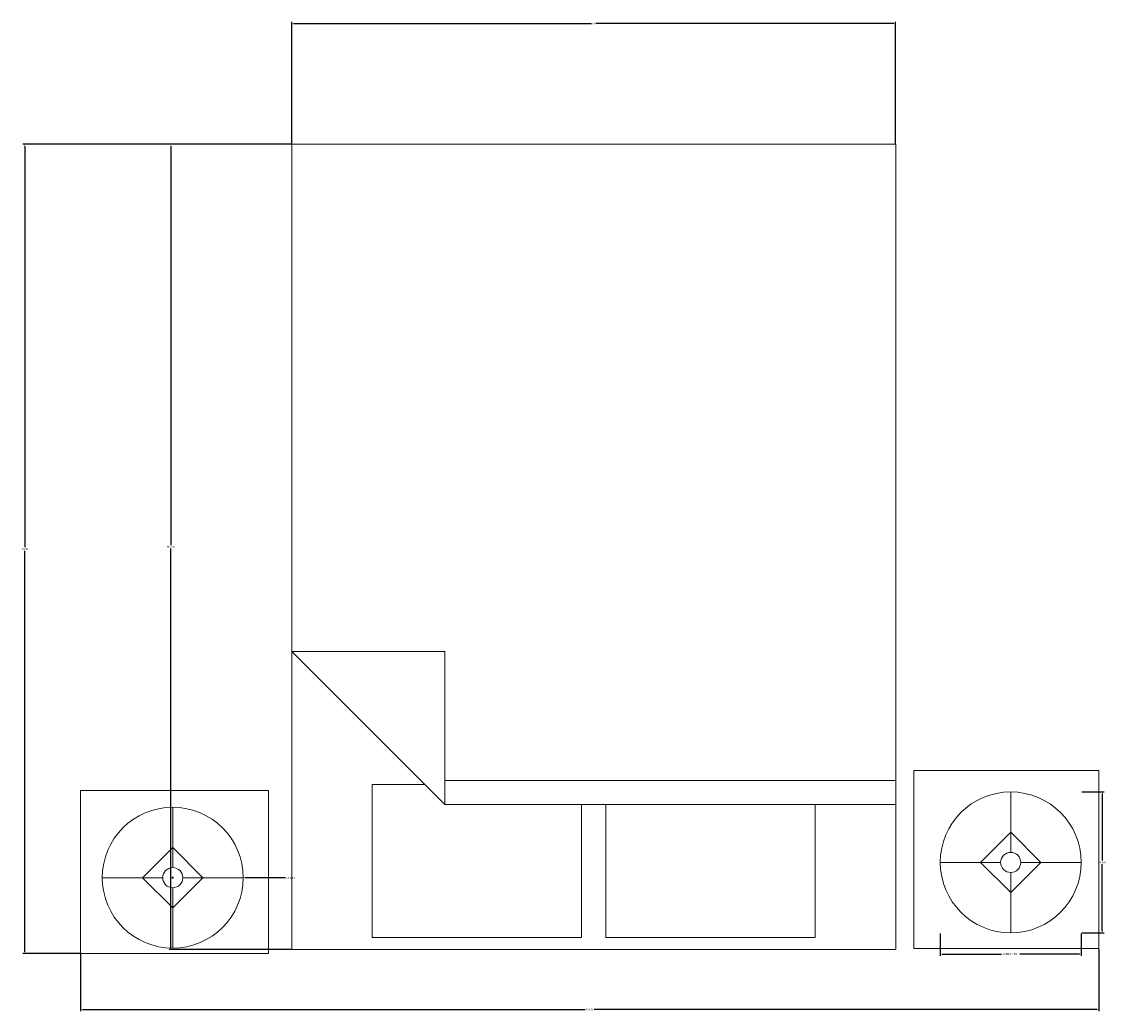
# Model space of a CAD drawing. Units: inches. Extents: x -52 to 1967, y 32 to 824.
# Tile 10 of 10: x 1859 to 1967, y 425 to 523. Entities that reach past the tile are written whole.
import ezdxf

# ---------------------------------------------------------------- set-up
doc = ezdxf.new("R2010")
doc.units = ezdxf.units.IN
doc.layers.add('A-ANNO-DIMS', color=2, linetype='Continuous', lineweight=18)
doc.layers.add('A-FURN', color=8, linetype='Continuous', lineweight=18)
doc.styles.get("Standard").update_dxf_attribs({"font": 'arial.ttf'})
doc.dimstyles.get("Standard").update_dxf_attribs({"dimtxt": 0.18, "dimasz": 0.18, "dimexe": 0.18, "dimexo": 0.0625, "dimgap": 0.09, "dimtad": 0, "dimtih": 1, "dimtoh": 1, "dimdec": 4, "dimzin": 0, "dimdsep": 46, "dimtxsty": 'Standard', "dimcen": 0.09, "dimadec": 0, "dimazin": 0, "dimtfac": 1, "dimtdec": 4, "dimtofl": 0, "dimtmove": 0, "dimatfit": 3, "dimfxl": 1, "dimtolj": 1, "dimtzin": 0, "dimarcsym": 0})

# ---------------------------------------------------------------- blocks, each defined once
blk = doc.blocks.new('Lamp - Table')
for p, q in [((0, 7), (0, 1)), ((0, 3), (-3, 0)), ((3, 0), (0, 3)), ((-1, 0), (-7, 0)), ((-3, 0), (0, -3)), ((0, -3), (3, 0)), ((1, 0), (7, 0)), ((0, -1), (0, -7))]:
    blk.add_line(p, q)
for radius in [7, 1]:
    blk.add_circle((0, 0), radius)
blk = doc.blocks.new('Bed - Queen')
for p, q in [((0, -80.00003), (0, 0)), ((0, 0), (59.99999, 0)), ((59.99999, 0), (59.99999, -80.00003)), ((7.99999, -1.2), (28.79998, -1.2)), ((7.99999, -14.4), (7.99999, -1.2)), ((28.79998, -1.2), (28.79998, -14.4)), ((31.19999, -1.2), (51.99999, -1.2)), ((31.19999, -14.4), (31.19999, -1.2)), ((51.99999, -1.2), (51.99999, -16.4)), ((0, -14.4), (44.8, -14.4)), ((59.99999, -29.6), (44.8, -14.4)), ((44.8, -14.4), (44.8, -29.6)), ((44.8, -16.8), (0, -16.8)), ((51.99999, -16.4), (46.79936, -16.4)), ((44.8, -29.6), (59.99999, -29.6)), ((59.99999, -80.00003), (0, -80.00003))]:
    blk.add_line(p, q)
blk = doc.blocks.new('*D29')
at = {"layer": 'A-ANNO-DIMS', "color": 0, "lineweight": -2, "transparency": 16777216}
for p, q in [((1885.95, 510.77), (1873.83, 510.77)), ((1874.01, 510.59), (1874.01, 470.95)), ((1874.01, 430.95), (1874.01, 470.59)), ((1885.95, 430.77), (1873.83, 430.77))]:
    blk.add_line(p, q, dxfattribs=at)
at = {"layer": 'A-ANNO-DIMS', "color": 0, "transparency": 16777216}
for points in [[(1873.98, 510.59), (1874.04, 510.59), (1874.01, 510.77)], [(1873.98, 430.95), (1874.04, 430.95), (1874.01, 430.77)]]:
    blk.add_solid(points, dxfattribs=at)
at = {"layer": 'Defpoints', "color": 0, "transparency": 16777216}
for p in [(1886.01, 510.77), (1874.01, 430.77), (1886.01, 430.77)]:
    blk.add_point(p, dxfattribs=at)
at = {"layer": 'A-ANNO-DIMS', "color": 0, "transparency": 16777216, "insert": (1874.01, 470.77), "char_height": 0.18, "attachment_point": 5}
blk.add_mtext('\\A1;BED 80', dxfattribs=at)
blk = doc.blocks.new('*D30')
at = {"layer": 'A-ANNO-DIMS', "color": 0, "lineweight": -2, "transparency": 16777216}
for p, q in [((1886.01, 510.83), (1886.01, 522.95)), ((1886.19, 522.77), (1915.79, 522.77)), ((1945.83, 522.77), (1916.23, 522.77)), ((1946.01, 510.83), (1946.01, 522.95))]:
    blk.add_line(p, q, dxfattribs=at)
at = {"layer": 'A-ANNO-DIMS', "color": 0, "transparency": 16777216}
for points in [[(1886.19, 522.8), (1886.19, 522.74), (1886.01, 522.77)], [(1945.83, 522.8), (1945.83, 522.74), (1946.01, 522.77)]]:
    blk.add_solid(points, dxfattribs=at)
at = {"layer": 'Defpoints', "color": 0, "transparency": 16777216}
for p in [(1886.01, 522.77), (1886.01, 510.77), (1946.01, 510.77)]:
    blk.add_point(p, dxfattribs=at)
at = {"layer": 'A-ANNO-DIMS', "color": 0, "transparency": 16777216, "insert": (1916.01, 522.77), "char_height": 0.18, "attachment_point": 5}
blk.add_mtext('\\A1;60', dxfattribs=at)
blk = doc.blocks.new('*D31')
at = {"layer": 'A-ANNO-DIMS', "color": 0, "lineweight": -2, "transparency": 16777216}
for p, q in [((1950.44, 432.35), (1950.44, 430.13)), ((1964.44, 432.35), (1964.44, 430.13)), ((1950.62, 430.31), (1956.54, 430.31)), ((1964.26, 430.31), (1958.34, 430.31))]:
    blk.add_line(p, q, dxfattribs=at)
at = {"layer": 'A-ANNO-DIMS', "color": 0, "transparency": 16777216}
for points in [[(1950.62, 430.34), (1950.62, 430.28), (1950.44, 430.31)], [(1964.26, 430.34), (1964.26, 430.28), (1964.44, 430.31)]]:
    blk.add_solid(points, dxfattribs=at)
at = {"layer": 'Defpoints', "color": 0, "transparency": 16777216}
for p in [(1950.44, 432.41), (1964.44, 432.41), (1964.44, 430.31)]:
    blk.add_point(p, dxfattribs=at)
at = {"layer": 'A-ANNO-DIMS', "color": 0, "transparency": 16777216, "insert": (1957.44, 430.31), "char_height": 0.18, "attachment_point": 5}
blk.add_mtext('\\A1;LAMP 14 TYP.', dxfattribs=at)
blk = doc.blocks.new('*D32')
at = {"layer": 'A-ANNO-DIMS', "color": 0, "lineweight": -2, "transparency": 16777216}
for p, q in [((1964.5, 446.41), (1966.72, 446.41)), ((1966.54, 446.23), (1966.54, 439.59)), ((1966.54, 432.59), (1966.54, 439.23)), ((1964.5, 432.41), (1966.72, 432.41))]:
    blk.add_line(p, q, dxfattribs=at)
at = {"layer": 'A-ANNO-DIMS', "color": 0, "transparency": 16777216}
for points in [[(1966.51, 446.23), (1966.57, 446.23), (1966.54, 446.41)], [(1966.51, 432.59), (1966.57, 432.59), (1966.54, 432.41)]]:
    blk.add_solid(points, dxfattribs=at)
at = {"layer": 'Defpoints', "color": 0, "transparency": 16777216}
for p in [(1964.44, 446.41), (1966.54, 446.41), (1964.44, 432.41)]:
    blk.add_point(p, dxfattribs=at)
at = {"layer": 'A-ANNO-DIMS', "color": 0, "transparency": 16777216, "insert": (1966.54, 439.41), "char_height": 0.18, "attachment_point": 5}
blk.add_mtext('\\A1;14 TYP.', dxfattribs=at)
blk = doc.blocks.new('*D130')
at = {"layer": 'A-ANNO-DIMS', "color": 0, "lineweight": -2, "transparency": 16777216}
for p, q in [((1865.04, 430.29), (1865.04, 424.62)), ((1966.2, 430.81), (1966.2, 424.62)), ((1865.22, 424.8), (1915.16, 424.8)), ((1966.02, 424.8), (1916.07, 424.8))]:
    blk.add_line(p, q, dxfattribs=at)
at = {"layer": 'A-ANNO-DIMS', "color": 0, "transparency": 16777216}
for points in [[(1865.22, 424.83), (1865.22, 424.77), (1865.04, 424.8)], [(1966.02, 424.83), (1966.02, 424.77), (1966.2, 424.8)]]:
    blk.add_solid(points, dxfattribs=at)
at = {"layer": 'Defpoints', "color": 0, "transparency": 16777216}
for p in [(1865.04, 430.35), (1966.2, 430.87), (1966.2, 424.8)]:
    blk.add_point(p, dxfattribs=at)
at = {"layer": 'A-ANNO-DIMS', "color": 0, "transparency": 16777216, "insert": (1915.62, 424.8), "char_height": 0.18, "attachment_point": 5}
blk.add_mtext('\\A1;101.16', dxfattribs=at)
blk = doc.blocks.new('*D131')
at = {"layer": 'A-ANNO-DIMS', "color": 0, "lineweight": -2, "transparency": 16777216}
for p, q in [((1885.95, 510.77), (1859.31, 510.77)), ((1859.49, 510.59), (1859.49, 470.74)), ((1859.49, 430.53), (1859.49, 470.38)), ((1864.98, 430.35), (1859.31, 430.35))]:
    blk.add_line(p, q, dxfattribs=at)
at = {"layer": 'A-ANNO-DIMS', "color": 0, "transparency": 16777216}
for points in [[(1859.46, 510.59), (1859.52, 510.59), (1859.49, 510.77)], [(1859.46, 430.53), (1859.52, 430.53), (1859.49, 430.35)]]:
    blk.add_solid(points, dxfattribs=at)
at = {"layer": 'Defpoints', "color": 0, "transparency": 16777216}
for p in [(1886.01, 510.77), (1859.49, 430.35), (1865.04, 430.35)]:
    blk.add_point(p, dxfattribs=at)
at = {"layer": 'A-ANNO-DIMS', "color": 0, "transparency": 16777216, "insert": (1859.49, 470.56), "char_height": 0.18, "attachment_point": 5}
blk.add_mtext('\\A1;80.42', dxfattribs=at)
blk = doc.blocks.new('*D161')
at = {"layer": 'A-ANNO-DIMS', "color": 0, "lineweight": -2, "transparency": 16777216}
for p, q in [((1874.1, 437.9), (1874.28, 437.9)), ((1874.19, 437.81), (1874.19, 437.99)), ((1885.39, 437.89), (1881.37, 437.89))]:
    blk.add_line(p, q, dxfattribs=at)
at = {"layer": 'A-ANNO-DIMS', "color": 0, "transparency": 16777216}
blk.add_solid([(1881.37, 437.92), (1881.37, 437.86), (1881.19, 437.89)], dxfattribs=at)
at = {"layer": 'Defpoints', "color": 0, "transparency": 16777216}
for p in [(1867.19, 437.9), (1881.19, 437.89)]:
    blk.add_point(p, dxfattribs=at)
at = {"layer": 'A-ANNO-DIMS', "color": 0, "transparency": 16777216, "insert": (1885.9, 437.89), "char_height": 0.18, "attachment_point": 5}
blk.add_mtext('\\A1;2X ∅14', dxfattribs=at)

msp = doc.modelspace()

# ---------------------------------------------------------------- linework, layer by layer
at = {"layer": 'A-FURN'}
for points in [[(1947.8059, 448.5534), (1966.1965, 448.5534), (1966.1965, 430.8688), (1947.8059, 430.8688)], [(1883.691, 430.3492), (1865.0393, 430.3492), (1865.0393, 446.572), (1883.691, 446.572)]]:
    msp.add_lwpolyline(points, close=True, dxfattribs=at)

# ---------------------------------------------------------------- block references
at = {"layer": 'A-FURN', "rotation": 180}
msp.add_blockref('Bed - Queen', (1946.0113, 430.768), dxfattribs=at)
at = {"layer": 'A-FURN'}
for p in [(1957.4408, 439.4144), (1874.1888, 437.8953)]:
    msp.add_blockref('Lamp - Table', p, dxfattribs=at)

# ---------------------------------------------------------------- dimensions: what is measured, and where the dimension line sits
at = {"layer": 'A-ANNO-DIMS'}
for base, p1, p2, angle, override, picture, middle in [((1886.0113, 522.768), (1946.0113, 510.768), (1886.0113, 510.768), 180, {"dimdec": 0, "dimlfac": 1, "dimrnd": 0, "dimzin": 0, "dimdsep": 46, "dimlunit": 2}, '*D30', (1916.0113, 522.768)), ((1859.4893, 430.3492), (1886.0113, 510.768), (1865.0393, 430.3492), 90, {"dimdec": 2, "dimlfac": 1, "dimrnd": 0, "dimzin": 0, "dimdsep": 46, "dimlunit": 2}, '*D131', (1859.4893, 470.5586))]:
    dim = msp.add_linear_dim(base=base, p1=p1, p2=p2, angle=angle, dimstyle='Standard', override=override, dxfattribs=at)
    dim.commit()
    dim.dimension.update_dxf_attribs({"geometry": picture, "text_midpoint": middle})
for base, p1, p2, angle, text, picture, middle in [((1874.0113, 430.768), (1886.0113, 510.768), (1886.0113, 430.768), 270, 'BED <>', '*D29', (1874.0113, 470.768)), ((1966.5408, 446.4144), (1964.4408, 432.4144), (1964.4408, 446.4144), 90, '<> TYP.', '*D32', (1966.5408, 439.4144))]:
    dim = msp.add_linear_dim(base=base, p1=p1, p2=p2, angle=angle, text=text, dimstyle='Standard', override={"dimdec": 0, "dimlfac": 1, "dimrnd": 0, "dimzin": 0, "dimdsep": 46, "dimlunit": 2}, dxfattribs=at)
    dim.commit()
    dim.dimension.update_dxf_attribs({"geometry": picture, "text_midpoint": middle})
dim = msp.add_diameter_dim_2p(p1=(1867.1888, 437.8956), p2=(1881.1888, 437.895), text='2X <>', dimstyle='Standard', override={"dimdec": 0, "dimlfac": 1, "dimrnd": 0, "dimzin": 0, "dimdsep": 46, "dimlunit": 2}, dxfattribs=at)
dim.commit()
dim.dimension.update_dxf_attribs({"geometry": '*D161', "text_midpoint": (1885.3888, 437.8948), "dimtype": 163})
dim = msp.add_linear_dim(base=(1964.4408, 430.3144), p1=(1950.4408, 432.4144), p2=(1964.4408, 432.4144), text='LAMP <> TYP.', dimstyle='Standard', override={"dimdec": 0, "dimlfac": 1, "dimrnd": 0, "dimzin": 0, "dimdsep": 46, "dimlunit": 2}, dxfattribs=at)
dim.commit()
dim.dimension.update_dxf_attribs({"geometry": '*D31', "text_midpoint": (1957.4408, 430.3144)})
dim = msp.add_linear_dim(base=(1966.1965, 424.7992), p1=(1865.0393, 430.3492), p2=(1966.1965, 430.8688), dimstyle='Standard', override={"dimdec": 2, "dimlfac": 1, "dimrnd": 0, "dimzin": 0, "dimdsep": 46, "dimlunit": 2}, dxfattribs=at)
dim.commit()
dim.dimension.update_dxf_attribs({"geometry": '*D130', "text_midpoint": (1915.6179, 424.7992)})

doc.saveas('drawing.dxf')
